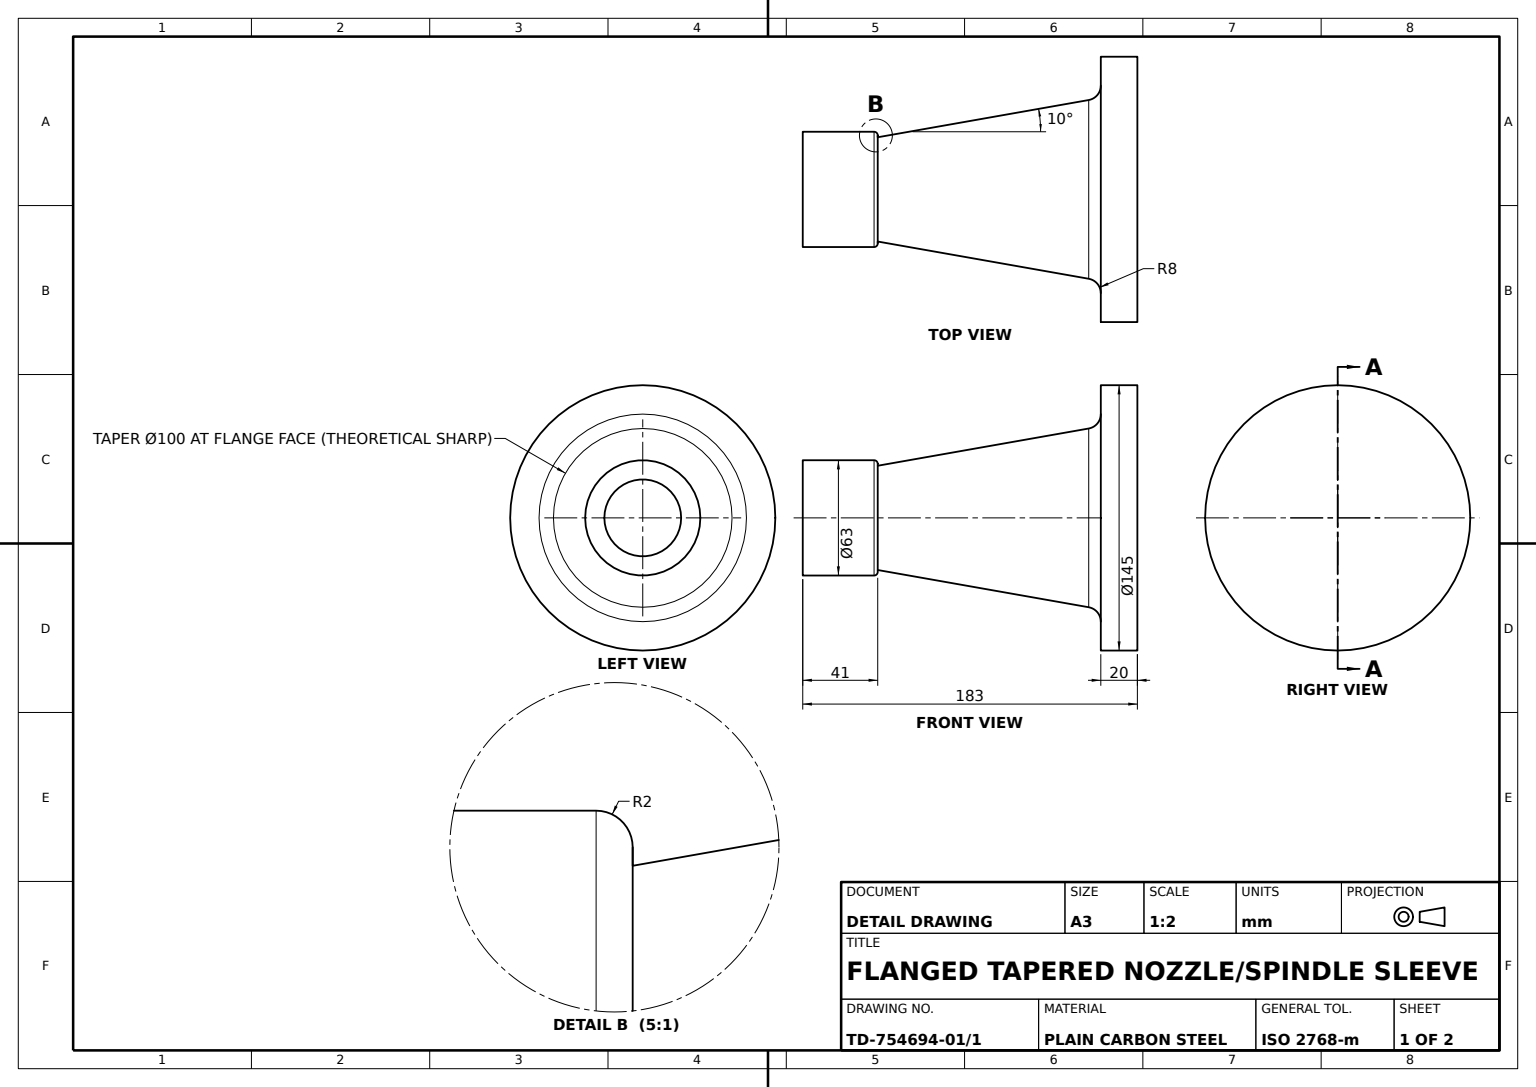
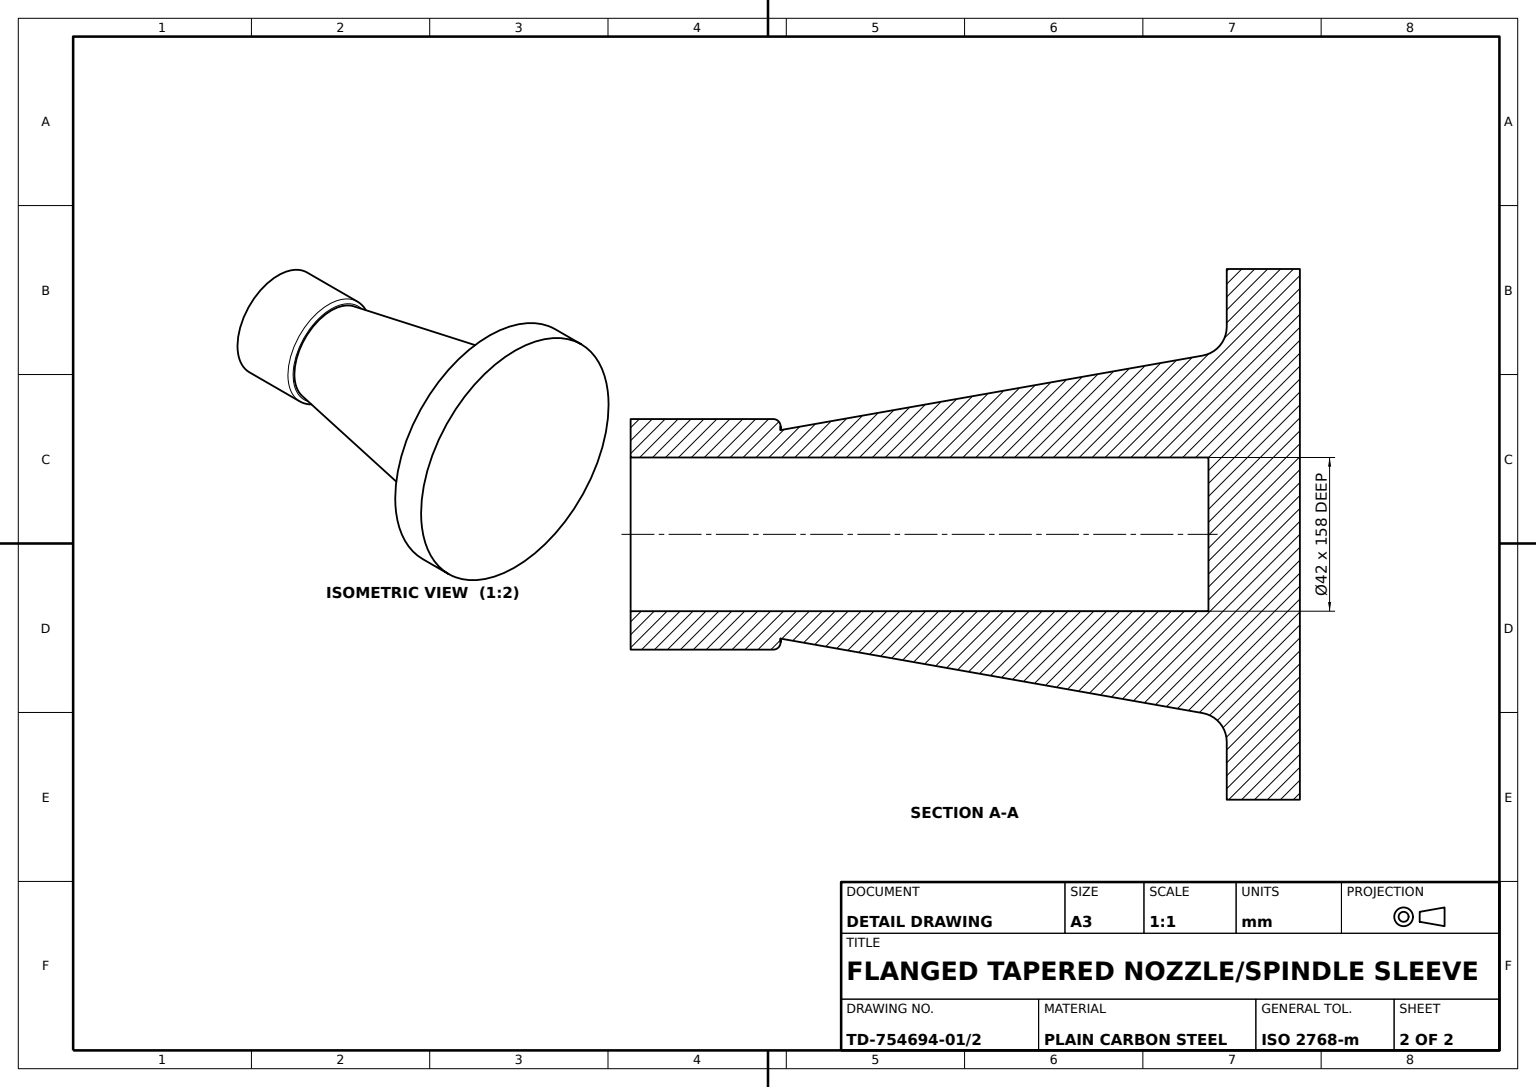
from build123d import *

# Parameters (mm, degrees)
FLANGE_SKETCH_145_R                = 72.5
FLANGE_145X20_DEPTH                = 20
TAPER_SKETCH_100_R                 = 50
TAPERED_BODY_100_10DEG_DRAFT_DEPTH = 125
TAPERED_BODY_100_10DEG_DRAFT_TAPER = 10
SPIGOT_63X38_DEPTH                 = 38
SPIGOT_63X38_DEPTH_BACK            = 3
SPIGOT_SKETCH_63_R                 = 31.5
BORE_SKETCH_42_R                   = 21
BORE_42X158_DEPTH                  = 158
FLANGE_ROOT_FILLET_R8_R            = 8
SPIGOT_EDGE_FILLET_R2_R            = 2


with BuildPart() as part:
    # Flange Sketch Ø145 → Flange Ø145x20 (new body)
    with BuildSketch(Plane.XY):
        Circle(FLANGE_SKETCH_145_R)
    extrude(amount=FLANGE_145X20_DEPTH)

    # Taper Sketch Ø100 → Tapered Body Ø100 10deg Draft (add)
    with BuildSketch(Plane.XY.offset(20)):
        Circle(TAPER_SKETCH_100_R)
    extrude(amount=TAPERED_BODY_100_10DEG_DRAFT_DEPTH, taper=TAPERED_BODY_100_10DEG_DRAFT_TAPER)

    # Spigot Sketch Ø63 → Spigot Ø63x38 (add, two sides: drawn at the far end of the back side and taken through both)
    with BuildSketch(Plane.XY.offset(145).offset(-SPIGOT_63X38_DEPTH_BACK)):
        Circle(SPIGOT_SKETCH_63_R)
    extrude(amount=SPIGOT_63X38_DEPTH + SPIGOT_63X38_DEPTH_BACK)

    # Bore Sketch Ø42 → Bore Ø42x158 (cut)
    with BuildSketch(Plane.XY.offset(183)):
        Circle(BORE_SKETCH_42_R)
    extrude(amount=-BORE_42X158_DEPTH, mode=Mode.SUBTRACT)

    # Flange Root Fillet R8
    flange_root_fillet_r8_edges = [part.edges().sort_by_distance(p)[0] for p in [
        (-50, 0, 20),
    ]]
    fillet(flange_root_fillet_r8_edges, radius=FLANGE_ROOT_FILLET_R8_R)

    # Spigot Edge Fillet R2
    spigot_edge_fillet_r2_edges = [part.edges().sort_by_distance(p)[0] for p in [
        (-31.5, 0, 142),
    ]]
    fillet(spigot_edge_fillet_r2_edges, radius=SPIGOT_EDGE_FILLET_R2_R)


solid = part.part
